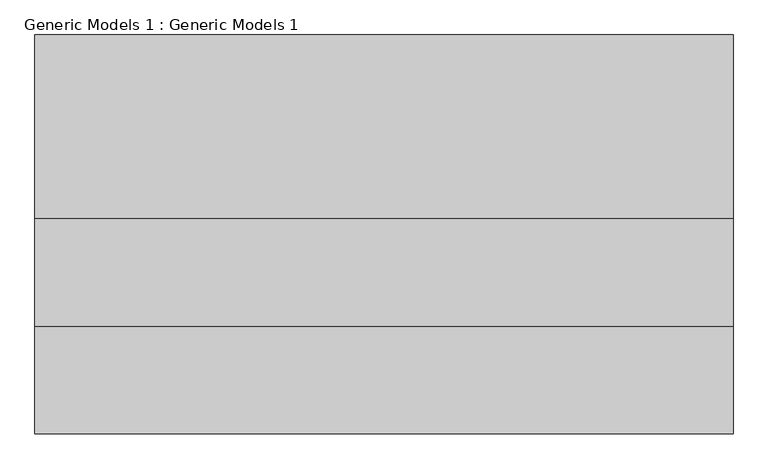
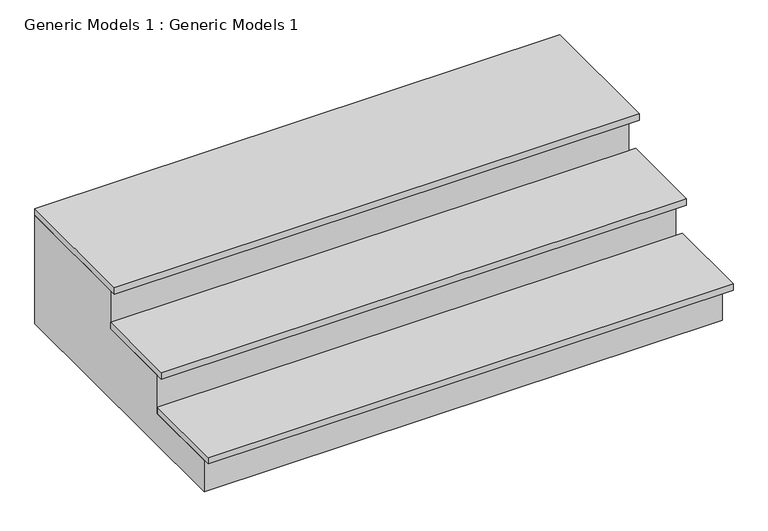
"""IFC4 building model written with IfcOpenShell, lengths in millimetres: proxy geometry, Generic Models 1 : Generic Models 1."""

from ifc_helpers import new_model, si_unit, frame, origin, place, context, project, spatial, polyline, outline, extrude, source, transform, mapped, element, save


def generic_models_1_generic_models_1_70b2dbcb(model_context):
    return source(origin(), model_context, "Body", "SweptSolid", [
        extrude(outline(polyline([(-6438.5842407, 3753.3127283), (-6438.5842407, 3234.9940862), (-8412.5002526, 3234.9940862), (-8412.5002526, 3753.3127283), (-6438.5842407, 3753.3127283)])), frame((0.0, 0.0, -25.4), z_axis=(0.0, 0.0, 1.0), x_axis=(1.0, 0.0, 0.0)), (0.0, 0.0, 1.0), 25.4),
        extrude(outline(polyline([(-6438.5842407, 3260.3940862), (-6438.5842407, 2930.1940862), (-8412.5002526, 2930.1940862), (-8412.5002526, 3260.3940862), (-6438.5842407, 3260.3940862)])), frame((0.0, 0.0, -177.8), z_axis=(0.0, 0.0, 1.0), x_axis=(1.0, 0.0, 0.0)), (0.0, 0.0, 1.0), 25.4),
        extrude(outline(polyline([(-6438.5842407, 2955.5940862), (-6438.5842407, 2625.3940862), (-8412.5002526, 2625.3940862), (-8412.5002526, 2955.5940862), (-6438.5842407, 2955.5940862)])), frame((0.0, 0.0, -330.2), z_axis=(0.0, 0.0, 1.0), x_axis=(1.0, 0.0, 0.0)), (0.0, 0.0, 1.0), 25.4),
        extrude(outline(polyline([(2650.7940862, -330.2), (2955.5940862, -330.2), (2955.5940862, -177.8), (3260.3940862, -177.8), (3260.3940862, -25.4), (3753.3127283, -25.4), (3753.3127283, -457.2), (2650.7940862, -457.2), (2650.7940862, -330.2)])), frame((-8412.5002526, 0.0, 0.0), z_axis=(1.0, 0.0, 0.0), x_axis=(0.0, 1.0, 0.0)), (0.0, 0.0, 1.0), 1948.5160119),
    ])


if __name__ == "__main__":
    model = new_model("IFC4")
    model_context = context("Model", 3, world=origin())
    ifc_project = project(units=[si_unit("LENGTHUNIT", "METRE", prefix="MILLI")], contexts=[model_context])
    site = spatial("IfcSite", under=ifc_project)
    building = spatial("IfcBuilding", under=site)
    placement = place(None, origin())
    generic_models_1_generic_models_1_shape = generic_models_1_generic_models_1_70b2dbcb(model_context)
    element("IfcBuildingElementProxy", 1, Name="Generic Models 1 : Generic Models 1", ObjectType="Generic Models 1 : Generic Models 1", at=placement, inside=building, context=model_context, shape_type="MappedRepresentation", body=[
        mapped(generic_models_1_generic_models_1_shape, transform((0.0, 0.0, 0.0), x_axis=(1.0, 0.0, 0.0), y_axis=(0.0, 1.0, 0.0), z_axis=(0.0, 0.0, 1.0))),
    ])
    save(model, "model.ifc")

# Revit data of these elements
# Element 1 (IfcBuildingElementProxy, "Generic Models 1 : Generic Models 1")
#   Materials on its faces: "BLACK GRANITE"
# Materials
#   "BLACK GRANITE": class "Generic", colour RGB 42 42 42, transparency 0, Cost = 0
